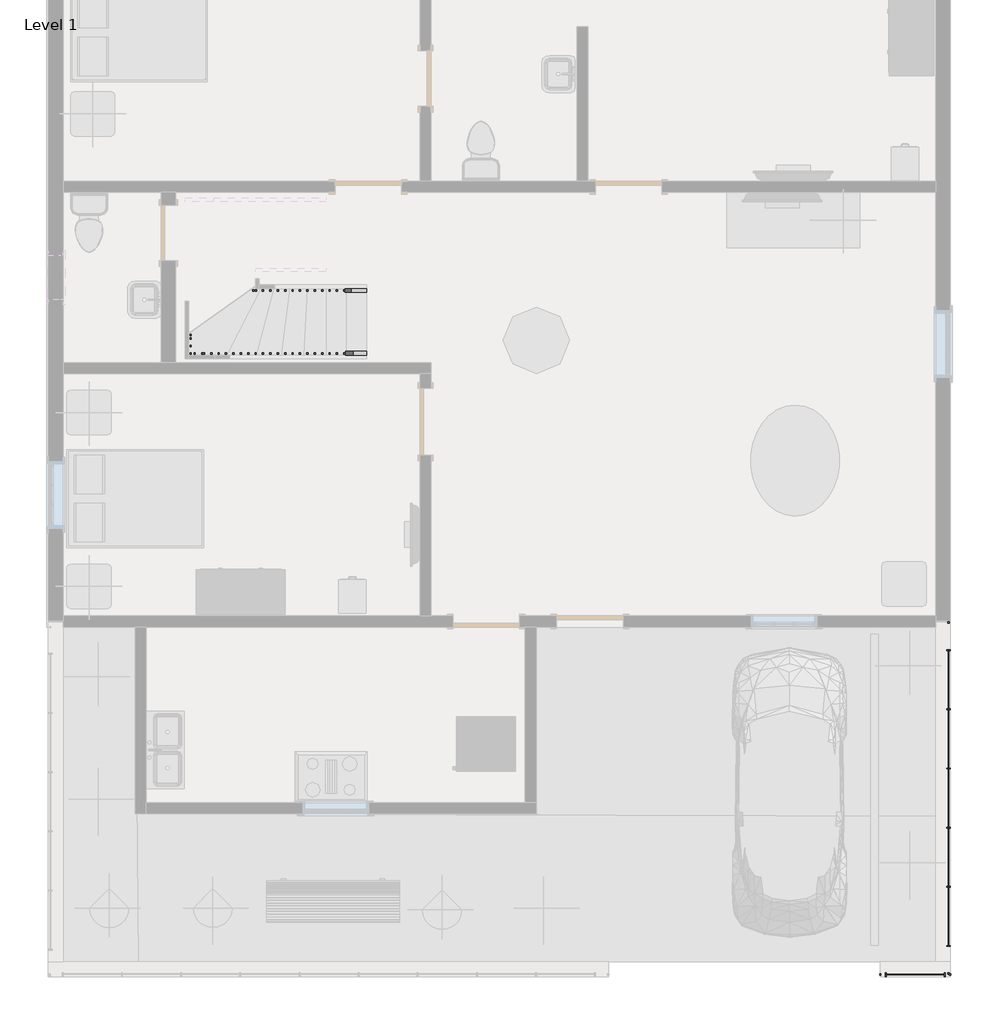
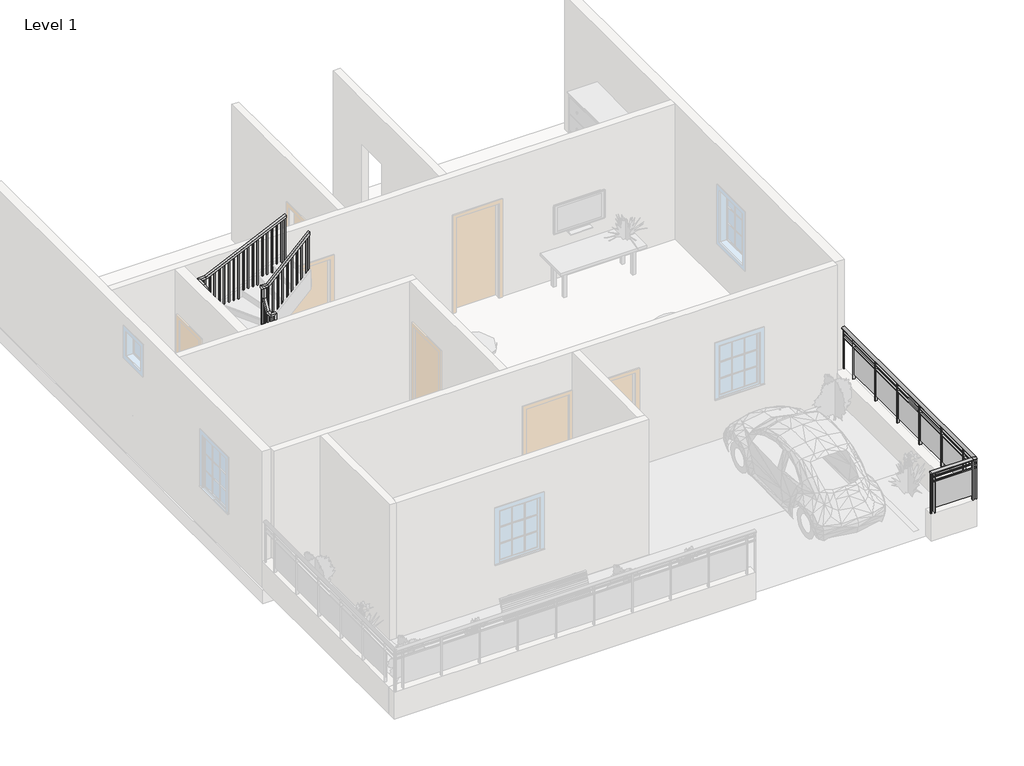
# One storey, part 2 of 3: 4 railings.
"""IFC4 building model written with IfcOpenShell, lengths in millimetres."""

from ifc_helpers import new_model, si_unit, point, frame, origin, place, context, project, spatial, polyline, ellipse_curve, trimmed, outline, extrude, faceted_brep, element, save
from ifc_brep_helpers import plane_surface, extruded_surface, advanced_brep

model = new_model("IFC4")

# Units and contexts
model_context = context("Model", 3, world=origin())
ifc_project = project(units=[si_unit("LENGTHUNIT", "METRE", prefix="MILLI")], contexts=[model_context])

# Site, building, storey
site = spatial("IfcSite", under=ifc_project)
building = spatial("IfcBuilding", under=site)
storey = spatial("IfcBuildingStorey", under=building, Name="Level 1", Elevation=0.0)

# Railings
placement = place(None, origin())
element("IfcRailing", 1, ObjectType="Glass Panel - Bottom Fill", at=placement, inside=storey, context=model_context, shape_type="SolidModel", body=[
    advanced_brep(
    [(-2180.6402453, -2817.8883114, 1524.0), (-2180.6402453, -2894.0883114, 1524.0), (-1215.4402453, -2817.8883114, 1524.0), (-1215.4402453, -2894.0883114, 1524.0)],
    [
        (0, 1, ellipse_curve(frame((-2180.6402453, -2855.9883114, 1524.0), z_axis=(-1.0, 0.0, 0.0), x_axis=(0.0, -1.0, 0.0)), 38.1, 28.575)),
        (1, 0, ellipse_curve(frame((-2180.6402453, -2855.9883114, 1524.0), z_axis=(-1.0, 0.0, 0.0), x_axis=(0.0, -1.0, 0.0)), 38.1, 28.575)),
        (2, 3, ellipse_curve(frame((-1215.4402453, -2855.9883114, 1524.0), z_axis=(1.0, 0.0, 0.0), x_axis=(0.0, -1.0, 0.0)), 38.1, 28.575)),
        (3, 2, ellipse_curve(frame((-1215.4402453, -2855.9883114, 1524.0), z_axis=(1.0, 0.0, 0.0), x_axis=(0.0, -1.0, 0.0)), 38.1, 28.575)),
        (0, 2),
        (3, 1),
    ],
    [
        plane_surface(frame((-2180.6402453, -2855.9883114, 1524.0), z_axis=(-1.0, 0.0, 0.0), x_axis=(0.0, 1.0, 0.0))),
        plane_surface(frame((-1215.4402453, -2855.9883114, 1524.0), z_axis=(1.0, 0.0, 0.0), x_axis=(0.0, 1.0, 0.0))),
        extruded_surface(trimmed(ellipse_curve(frame((-1215.4402453, -2855.9883114, 1524.0), z_axis=(-1.0, 0.0, 0.0), x_axis=(0.0, -1.0, 0.0)), 38.1, 28.575), [point((-1215.4402453, -2817.8883114, 1524.0))], [point((-1215.4402453, -2894.0883114, 1524.0))], True, "CARTESIAN"), (-965.2, 0.0, 0.0), 965.2),
        extruded_surface(trimmed(ellipse_curve(frame((-1215.4402453, -2855.9883114, 1524.0), z_axis=(-1.0, 0.0, 0.0), x_axis=(0.0, -1.0, 0.0)), 38.1, 28.575), [point((-1215.4402453, -2894.0883114, 1524.0))], [point((-1215.4402453, -2817.8883114, 1524.0))], True, "CARTESIAN"), (-965.2, 0.0, 0.0), 965.2),
    ],
    [
        (0, [[1, 2]]),
        (1, [[3, 4]]),
        (2, [[-1, 5, -4, 6]]),
        (3, [[-2, -6, -3, -5]]),
    ],
),
    extrude(outline(polyline([(-2180.6402453, -2868.6883114), (-2180.6402453, -2843.2883114), (-1215.4402453, -2843.2883114), (-1215.4402453, -2868.6883114), (-2180.6402453, -2868.6883114)])), frame((0.0, 0.0, 1409.7), z_axis=(0.0, 0.0, 1.0), x_axis=(1.0, 0.0, 0.0)), (0.0, 0.0, 1.0), 25.4),
    extrude(outline(polyline([(-2180.6402453, -2868.6883114), (-2180.6402453, -2843.2883114), (-1215.4402453, -2843.2883114), (-1215.4402453, -2868.6883114), (-2180.6402453, -2868.6883114)])), frame((0.0, 0.0, 1308.1), z_axis=(0.0, 0.0, 1.0), x_axis=(1.0, 0.0, 0.0)), (0.0, 0.0, 1.0), 25.4),
    extrude(outline(polyline([(-1297.9902453, -2881.3883114), (-1297.9902453, -2830.5883114), (-1285.2902453, -2830.5883114), (-1285.2902453, -2881.3883114), (-1297.9902453, -2881.3883114)])), frame((0.0, 0.0, 609.6), z_axis=(0.0, 0.0, 1.0), x_axis=(1.0, 0.0, 0.0)), (0.0, 0.0, 1.0), 885.6788223),
    extrude(outline(polyline([(-2104.4402453, -2849.4531544), (-1291.6402453, -2849.4531544), (-1291.6402453, -2855.8031544), (-2104.4402453, -2855.8031544), (-2104.4402453, -2849.4531544)])), frame((0.0, 0.0, 711.2), z_axis=(0.0, 0.0, 1.0), x_axis=(1.0, 0.0, 0.0)), (0.0, 0.0, 1.0), 596.9),
    extrude(outline(polyline([(-2110.7902453, -2881.3883114), (-2110.7902453, -2830.5883114), (-2098.0902453, -2830.5883114), (-2098.0902453, -2881.3883114), (-2110.7902453, -2881.3883114)])), frame((0.0, 0.0, 609.6), z_axis=(0.0, 0.0, 1.0), x_axis=(1.0, 0.0, 0.0)), (0.0, 0.0, 1.0), 885.6788223),
    extrude(outline(polyline([(-1228.1402453, -2865.5133114), (-1228.1402453, -2846.4633114), (-1209.0902453, -2846.4633114), (-1209.0902453, -2865.5133114), (-1228.1402453, -2865.5133114)])), frame((0.0, 0.0, 609.6), z_axis=(0.0, 0.0, 1.0), x_axis=(1.0, 0.0, 0.0)), (0.0, 0.0, 1.0), 885.6788223),
    extrude(outline(polyline([(-2186.9902453, -2865.5133114), (-2186.9902453, -2846.4633114), (-2167.9402453, -2846.4633114), (-2167.9402453, -2865.5133114), (-2186.9902453, -2865.5133114)])), frame((0.0, 0.0, 609.6), z_axis=(0.0, 0.0, 1.0), x_axis=(1.0, 0.0, 0.0)), (0.0, 0.0, 1.0), 885.6788223),
])
element("IfcRailing", 2, ObjectType="Glass Panel - Bottom Fill", at=placement, inside=storey, context=model_context, shape_type="SolidModel", body=[
    advanced_brep(
    [(-1202.7402453, 1982.7116886, 1524.0), (-1278.9402453, 1982.7116886, 1524.0), (-1202.7402453, -2843.2883114, 1524.0), (-1278.9402453, -2843.2883114, 1524.0)],
    [
        (0, 1, ellipse_curve(frame((-1240.8402453, 1982.7116886, 1524.0), z_axis=(0.0, 1.0, 0.0), x_axis=(-1.0, 0.0, 0.0)), 38.1, 28.575)),
        (1, 0, ellipse_curve(frame((-1240.8402453, 1982.7116886, 1524.0), z_axis=(0.0, 1.0, 0.0), x_axis=(-1.0, 0.0, 0.0)), 38.1, 28.575)),
        (2, 3, ellipse_curve(frame((-1240.8402453, -2843.2883114, 1524.0), z_axis=(0.0, -1.0, 0.0), x_axis=(-1.0, 0.0, 0.0)), 38.1, 28.575)),
        (3, 2, ellipse_curve(frame((-1240.8402453, -2843.2883114, 1524.0), z_axis=(0.0, -1.0, 0.0), x_axis=(-1.0, 0.0, 0.0)), 38.1, 28.575)),
        (0, 2),
        (3, 1),
    ],
    [
        plane_surface(frame((-1240.8402453, 1982.7116886, 1524.0), z_axis=(0.0, 1.0, 0.0), x_axis=(0.0, 0.0, -1.0))),
        plane_surface(frame((-1240.8402453, -2843.2883114, 1524.0), z_axis=(0.0, -1.0, 0.0), x_axis=(0.0, 0.0, -1.0))),
        extruded_surface(trimmed(ellipse_curve(frame((-1240.8402453, -2843.2883114, 1524.0), z_axis=(0.0, 1.0, 0.0), x_axis=(-1.0, 0.0, 0.0)), 38.1, 28.575), [point((-1202.7402453, -2843.2883114, 1524.0))], [point((-1278.9402453, -2843.2883114, 1524.0))], True, "CARTESIAN"), (0.0, 4826.0, 0.0), 4826.0),
        extruded_surface(trimmed(ellipse_curve(frame((-1240.8402453, -2843.2883114, 1524.0), z_axis=(0.0, 1.0, 0.0), x_axis=(-1.0, 0.0, 0.0)), 38.1, 28.575), [point((-1278.9402453, -2843.2883114, 1524.0))], [point((-1202.7402453, -2843.2883114, 1524.0))], True, "CARTESIAN"), (0.0, 4826.0, 0.0), 4826.0),
    ],
    [
        (0, [[1, 2]]),
        (1, [[3, 4]]),
        (2, [[-1, 5, -4, 6]]),
        (3, [[-2, -6, -3, -5]]),
    ],
),
    extrude(outline(polyline([(-1253.5402453, 1982.7116886), (-1228.1402453, 1982.7116886), (-1228.1402453, -2843.2883114), (-1253.5402453, -2843.2883114), (-1253.5402453, 1982.7116886)])), frame((0.0, 0.0, 1409.7), z_axis=(0.0, 0.0, 1.0), x_axis=(1.0, 0.0, 0.0)), (0.0, 0.0, 1.0), 25.4),
    extrude(outline(polyline([(-1253.5402453, 1982.7116886), (-1228.1402453, 1982.7116886), (-1228.1402453, -2843.2883114), (-1253.5402453, -2843.2883114), (-1253.5402453, 1982.7116886)])), frame((0.0, 0.0, 1308.1), z_axis=(0.0, 0.0, 1.0), x_axis=(1.0, 0.0, 0.0)), (0.0, 0.0, 1.0), 25.4),
    extrude(outline(polyline([(-1266.2402453, -2455.9383114), (-1215.4402453, -2455.9383114), (-1215.4402453, -2468.6383114), (-1266.2402453, -2468.6383114), (-1266.2402453, -2455.9383114)])), frame((0.0, 0.0, 609.6), z_axis=(0.0, 0.0, 1.0), x_axis=(1.0, 0.0, 0.0)), (0.0, 0.0, 1.0), 885.6788223),
    extrude(outline(polyline([(-1234.3050883, -1649.4883114), (-1234.3050883, -2462.2883114), (-1240.6550883, -2462.2883114), (-1240.6550883, -1649.4883114), (-1234.3050883, -1649.4883114)])), frame((0.0, 0.0, 711.2), z_axis=(0.0, 0.0, 1.0), x_axis=(1.0, 0.0, 0.0)), (0.0, 0.0, 1.0), 596.9),
    extrude(outline(polyline([(-1266.2402453, -1643.1383114), (-1215.4402453, -1643.1383114), (-1215.4402453, -1655.8383114), (-1266.2402453, -1655.8383114), (-1266.2402453, -1643.1383114)])), frame((0.0, 0.0, 609.6), z_axis=(0.0, 0.0, 1.0), x_axis=(1.0, 0.0, 0.0)), (0.0, 0.0, 1.0), 885.6788223),
    extrude(outline(polyline([(-1234.3050883, -836.6883114), (-1234.3050883, -1649.4883114), (-1240.6550883, -1649.4883114), (-1240.6550883, -836.6883114), (-1234.3050883, -836.6883114)])), frame((0.0, 0.0, 711.2), z_axis=(0.0, 0.0, 1.0), x_axis=(1.0, 0.0, 0.0)), (0.0, 0.0, 1.0), 596.9),
    extrude(outline(polyline([(-1266.2402453, -830.3383114), (-1215.4402453, -830.3383114), (-1215.4402453, -843.0383114), (-1266.2402453, -843.0383114), (-1266.2402453, -830.3383114)])), frame((0.0, 0.0, 609.6), z_axis=(0.0, 0.0, 1.0), x_axis=(1.0, 0.0, 0.0)), (0.0, 0.0, 1.0), 885.6788223),
    extrude(outline(polyline([(-1234.3050883, -23.8883114), (-1234.3050883, -836.6883114), (-1240.6550883, -836.6883114), (-1240.6550883, -23.8883114), (-1234.3050883, -23.8883114)])), frame((0.0, 0.0, 711.2), z_axis=(0.0, 0.0, 1.0), x_axis=(1.0, 0.0, 0.0)), (0.0, 0.0, 1.0), 596.9),
    extrude(outline(polyline([(-1266.2402453, -17.5383114), (-1215.4402453, -17.5383114), (-1215.4402453, -30.2383114), (-1266.2402453, -30.2383114), (-1266.2402453, -17.5383114)])), frame((0.0, 0.0, 609.6), z_axis=(0.0, 0.0, 1.0), x_axis=(1.0, 0.0, 0.0)), (0.0, 0.0, 1.0), 885.6788223),
    extrude(outline(polyline([(-1234.3050883, 788.9116886), (-1234.3050883, -23.8883114), (-1240.6550883, -23.8883114), (-1240.6550883, 788.9116886), (-1234.3050883, 788.9116886)])), frame((0.0, 0.0, 711.2), z_axis=(0.0, 0.0, 1.0), x_axis=(1.0, 0.0, 0.0)), (0.0, 0.0, 1.0), 596.9),
    extrude(outline(polyline([(-1266.2402453, 795.2616886), (-1215.4402453, 795.2616886), (-1215.4402453, 782.5616886), (-1266.2402453, 782.5616886), (-1266.2402453, 795.2616886)])), frame((0.0, 0.0, 609.6), z_axis=(0.0, 0.0, 1.0), x_axis=(1.0, 0.0, 0.0)), (0.0, 0.0, 1.0), 885.6788223),
    extrude(outline(polyline([(-1234.3050883, 1601.7116886), (-1234.3050883, 788.9116886), (-1240.6550883, 788.9116886), (-1240.6550883, 1601.7116886), (-1234.3050883, 1601.7116886)])), frame((0.0, 0.0, 711.2), z_axis=(0.0, 0.0, 1.0), x_axis=(1.0, 0.0, 0.0)), (0.0, 0.0, 1.0), 596.9),
    extrude(outline(polyline([(-1266.2402453, 1608.0616886), (-1215.4402453, 1608.0616886), (-1215.4402453, 1595.3616886), (-1266.2402453, 1595.3616886), (-1266.2402453, 1608.0616886)])), frame((0.0, 0.0, 609.6), z_axis=(0.0, 0.0, 1.0), x_axis=(1.0, 0.0, 0.0)), (0.0, 0.0, 1.0), 885.6788223),
    extrude(outline(polyline([(-1250.3652453, -2830.5883114), (-1231.3152453, -2830.5883114), (-1231.3152453, -2849.6383114), (-1250.3652453, -2849.6383114), (-1250.3652453, -2830.5883114)])), frame((0.0, 0.0, 609.6), z_axis=(0.0, 0.0, 1.0), x_axis=(1.0, 0.0, 0.0)), (0.0, 0.0, 1.0), 885.6788223),
    extrude(outline(polyline([(-1250.3652453, 1989.0616886), (-1231.3152453, 1989.0616886), (-1231.3152453, 1970.0116886), (-1250.3652453, 1970.0116886), (-1250.3652453, 1989.0616886)])), frame((0.0, 0.0, 609.6), z_axis=(0.0, 0.0, 1.0), x_axis=(1.0, 0.0, 0.0)), (0.0, 0.0, 1.0), 885.6788223),
])
element("IfcRailing", 3, ObjectType="Handrail - Rectangular", at=placement, inside=storey, context=model_context, shape_type="SolidModel", body=[
    faceted_brep([(-9238.1085535, 6516.6116886, 1025.2529681), (-9238.1085535, 6516.6116886, 959.7067088), (-9238.1085535, 6567.4116886, 959.7067088), (-9238.1085535, 6567.4116886, 1025.2529681), (-10689.6402453, 6516.6116886, 2208.7848338), (-10740.4402453, 6516.6116886, 2184.659247), (-10740.4402453, 6567.4116886, 2184.659247), (-10689.6402453, 6567.4116886, 2208.7848338), (-10689.6402453, 6516.6116886, 2414.6281882), (-10740.4402453, 6516.6116886, 2363.8281882), (-10740.4402453, 6567.4116886, 2363.8281882), (-10689.6402453, 6567.4116886, 2414.6281882), (-10816.6402453, 6516.6116886, 2414.6281882), (-10816.6402453, 6516.6116886, 2363.8281882), (-10765.8402453, 6567.4116886, 2363.8281882), (-10765.8402453, 6567.4116886, 2414.6281882), (-10816.6402453, 6643.6116886, 2414.6281882), (-10816.6402453, 6672.7330225, 2363.8281882), (-10765.8402453, 6672.7330225, 2363.8281882), (-10765.8402453, 6643.6116886, 2414.6281882), (-10816.6402453, 6770.6116886, 2631.5051451), (-10816.6402453, 6821.4116886, 2617.7256424), (-10765.8402453, 6821.4116886, 2617.7256424), (-10765.8402453, 6770.6116886, 2631.5051451), (-10816.6402453, 6770.6116886, 2849.930498), (-10816.6402453, 6821.4116886, 2799.130498), (-10765.8402453, 6821.4116886, 2799.130498), (-10765.8402453, 6770.6116886, 2849.930498), (-10816.6402453, 6897.6116886, 2849.930498), (-10816.6402453, 6897.6116886, 2799.130498), (-10765.8402453, 6846.8116886, 2799.130498), (-10765.8402453, 6846.8116886, 2849.930498), (-10689.6402453, 6897.6116886, 2849.930498), (-10668.8144223, 6897.6116886, 2799.130498), (-10668.8144223, 6846.8116886, 2799.130498), (-10689.6402453, 6846.8116886, 2849.930498), (-9796.9085535, 6897.6116886, 3729.7628764), (-9796.9085535, 6846.8116886, 3729.7628764), (-9796.9085535, 6846.8116886, 3658.4379712), (-9796.9085535, 6897.6116886, 3658.4379712)], [[[0, 1, 2, 3]], [[1, 0, 4, 5]], [[2, 1, 5, 6]], [[3, 2, 6, 7]], [[0, 3, 7, 4]], [[5, 4, 8, 9]], [[6, 5, 9, 10]], [[7, 6, 10, 11]], [[4, 7, 11, 8]], [[9, 8, 12, 13]], [[10, 9, 13, 14]], [[11, 10, 14, 15]], [[8, 11, 15, 12]], [[13, 12, 16, 17]], [[14, 13, 17, 18]], [[15, 14, 18, 19]], [[12, 15, 19, 16]], [[17, 16, 20, 21]], [[18, 17, 21, 22]], [[19, 18, 22, 23]], [[16, 19, 23, 20]], [[21, 20, 24, 25]], [[22, 21, 25, 26]], [[23, 22, 26, 27]], [[20, 23, 27, 24]], [[25, 24, 28, 29]], [[26, 25, 29, 30]], [[27, 26, 30, 31]], [[24, 27, 31, 28]], [[29, 28, 32, 33]], [[30, 29, 33, 34]], [[31, 30, 34, 35]], [[28, 31, 35, 32]], [[36, 37, 38, 39]], [[33, 32, 36, 39]], [[34, 33, 39, 38]], [[35, 34, 38, 37]], [[32, 35, 37, 36]]]),
    extrude(outline(polyline([(3616.6526879, -9839.3064551), (3597.8779463, -9858.3564551), (2540.0, -9858.3564551), (2540.0, -9839.3064551), (3616.6526879, -9839.3064551)])), frame((0.0, 6862.6866886, 0.0), z_axis=(0.0, 1.0, 0.0), x_axis=(0.0, 0.0, 1.0)), (0.0, 0.0, 1.0), 19.05),
    extrude(outline(polyline([(3516.5207329, -9940.9064551), (3497.7459913, -9959.9564551), (2540.0, -9959.9564551), (2540.0, -9940.9064551), (3516.5207329, -9940.9064551)])), frame((0.0, 6862.6866886, 0.0), z_axis=(0.0, 1.0, 0.0), x_axis=(0.0, 0.0, 1.0)), (0.0, 0.0, 1.0), 19.05),
    extrude(outline(polyline([(3416.3887778, -10042.5064551), (3397.6140362, -10061.5564551), (2540.0, -10061.5564551), (2540.0, -10042.5064551), (3416.3887778, -10042.5064551)])), frame((0.0, 6862.6866886, 0.0), z_axis=(0.0, 1.0, 0.0), x_axis=(0.0, 0.0, 1.0)), (0.0, 0.0, 1.0), 19.05),
    extrude(outline(polyline([(3316.2568227, -10144.1064551), (3297.4820812, -10163.1564551), (2370.6666667, -10163.1564551), (2370.6666667, -10144.1064551), (3316.2568227, -10144.1064551)])), frame((0.0, 6862.6866886, 0.0), z_axis=(0.0, 1.0, 0.0), x_axis=(0.0, 0.0, 1.0)), (0.0, 0.0, 1.0), 19.05),
    extrude(outline(polyline([(3216.1248677, -10245.7064551), (3197.3501261, -10264.7564551), (2370.6666667, -10264.7564551), (2370.6666667, -10245.7064551), (3216.1248677, -10245.7064551)])), frame((0.0, 6862.6866886, 0.0), z_axis=(0.0, 1.0, 0.0), x_axis=(0.0, 0.0, 1.0)), (0.0, 0.0, 1.0), 19.05),
    extrude(outline(polyline([(3115.9929126, -10347.3064551), (3097.218171, -10366.3564551), (2201.3333333, -10366.3564551), (2201.3333333, -10347.3064551), (3115.9929126, -10347.3064551)])), frame((0.0, 6862.6866886, 0.0), z_axis=(0.0, 1.0, 0.0), x_axis=(0.0, 0.0, 1.0)), (0.0, 0.0, 1.0), 19.05),
    extrude(outline(polyline([(3015.8609575, -10448.9064551), (2997.086216, -10467.9564551), (2201.3333333, -10467.9564551), (2201.3333333, -10448.9064551), (3015.8609575, -10448.9064551)])), frame((0.0, 6862.6866886, 0.0), z_axis=(0.0, 1.0, 0.0), x_axis=(0.0, 0.0, 1.0)), (0.0, 0.0, 1.0), 19.05),
    extrude(outline(polyline([(2915.7290025, -10550.5064551), (2896.9542609, -10569.5564551), (2032.0, -10569.5564551), (2032.0, -10550.5064551), (2915.7290025, -10550.5064551)])), frame((0.0, 6862.6866886, 0.0), z_axis=(0.0, 1.0, 0.0), x_axis=(0.0, 0.0, 1.0)), (0.0, 0.0, 1.0), 19.05),
    extrude(outline(polyline([(2815.5970474, -10652.1064551), (2796.8223058, -10671.1564551), (2032.0, -10671.1564551), (2032.0, -10652.1064551), (2815.5970474, -10652.1064551)])), frame((0.0, 6862.6866886, 0.0), z_axis=(0.0, 1.0, 0.0), x_axis=(0.0, 0.0, 1.0)), (0.0, 0.0, 1.0), 19.05),
    extrude(outline(polyline([(6750.4725924, 2496.5834745), (6769.5225924, 2529.115018), (6769.5225924, 1524.0), (6750.4725924, 1524.0), (6750.4725924, 2496.5834745)])), frame((-10800.7652453, 0.0, 0.0), z_axis=(1.0, 0.0, 0.0), x_axis=(0.0, 1.0, 0.0)), (0.0, 0.0, 1.0), 19.05),
    extrude(outline(polyline([(6648.8725924, 2323.0819089), (6667.9225924, 2355.6134525), (6667.9225924, 1524.0), (6648.8725924, 1524.0), (6648.8725924, 2323.0819089)])), frame((-10800.7652453, 0.0, 0.0), z_axis=(1.0, 0.0, 0.0), x_axis=(0.0, 1.0, 0.0)), (0.0, 0.0, 1.0), 19.05),
    extrude(outline(polyline([(2111.7191617, -10650.9835535), (2127.2519138, -10670.0335535), (1016.0, -10670.0335535), (1016.0, -10650.9835535), (2111.7191617, -10650.9835535)])), frame((0.0, 6532.4866886, 0.0), z_axis=(0.0, 1.0, 0.0), x_axis=(0.0, 0.0, 1.0)), (0.0, 0.0, 1.0), 19.05),
    extrude(outline(polyline([(2028.8778167, -10549.3835535), (2044.4105689, -10568.4335535), (1016.0, -10568.4335535), (1016.0, -10549.3835535), (2028.8778167, -10549.3835535)])), frame((0.0, 6532.4866886, 0.0), z_axis=(0.0, 1.0, 0.0), x_axis=(0.0, 0.0, 1.0)), (0.0, 0.0, 1.0), 19.05),
    extrude(outline(polyline([(1946.0364718, -10447.7835535), (1961.569224, -10466.8335535), (846.6666667, -10466.8335535), (846.6666667, -10447.7835535), (1946.0364718, -10447.7835535)])), frame((0.0, 6532.4866886, 0.0), z_axis=(0.0, 1.0, 0.0), x_axis=(0.0, 0.0, 1.0)), (0.0, 0.0, 1.0), 19.05),
    extrude(outline(polyline([(1863.1951269, -10346.1835535), (1878.7278791, -10365.2335535), (846.6666667, -10365.2335535), (846.6666667, -10346.1835535), (1863.1951269, -10346.1835535)])), frame((0.0, 6532.4866886, 0.0), z_axis=(0.0, 1.0, 0.0), x_axis=(0.0, 0.0, 1.0)), (0.0, 0.0, 1.0), 19.05),
    extrude(outline(polyline([(1780.353782, -10244.5835535), (1795.8865341, -10263.6335535), (677.3333333, -10263.6335535), (677.3333333, -10244.5835535), (1780.353782, -10244.5835535)])), frame((0.0, 6532.4866886, 0.0), z_axis=(0.0, 1.0, 0.0), x_axis=(0.0, 0.0, 1.0)), (0.0, 0.0, 1.0), 19.05),
    extrude(outline(polyline([(1697.5124371, -10142.9835535), (1713.0451892, -10162.0335535), (677.3333333, -10162.0335535), (677.3333333, -10142.9835535), (1697.5124371, -10142.9835535)])), frame((0.0, 6532.4866886, 0.0), z_axis=(0.0, 1.0, 0.0), x_axis=(0.0, 0.0, 1.0)), (0.0, 0.0, 1.0), 19.05),
    extrude(outline(polyline([(1614.6710921, -10041.3835535), (1630.2038443, -10060.4335535), (508.0, -10060.4335535), (508.0, -10041.3835535), (1614.6710921, -10041.3835535)])), frame((0.0, 6532.4866886, 0.0), z_axis=(0.0, 1.0, 0.0), x_axis=(0.0, 0.0, 1.0)), (0.0, 0.0, 1.0), 19.05),
    extrude(outline(polyline([(1531.8297472, -9939.7835535), (1547.3624994, -9958.8335535), (508.0, -9958.8335535), (508.0, -9939.7835535), (1531.8297472, -9939.7835535)])), frame((0.0, 6532.4866886, 0.0), z_axis=(0.0, 1.0, 0.0), x_axis=(0.0, 0.0, 1.0)), (0.0, 0.0, 1.0), 19.05),
    extrude(outline(polyline([(1448.9884023, -9838.1835535), (1464.5211545, -9857.2335535), (508.0, -9857.2335535), (508.0, -9838.1835535), (1448.9884023, -9838.1835535)])), frame((0.0, 6532.4866886, 0.0), z_axis=(0.0, 1.0, 0.0), x_axis=(0.0, 0.0, 1.0)), (0.0, 0.0, 1.0), 19.05),
    extrude(outline(polyline([(1366.1470574, -9736.5835535), (1381.6798095, -9755.6335535), (338.6666667, -9755.6335535), (338.6666667, -9736.5835535), (1366.1470574, -9736.5835535)])), frame((0.0, 6532.4866886, 0.0), z_axis=(0.0, 1.0, 0.0), x_axis=(0.0, 0.0, 1.0)), (0.0, 0.0, 1.0), 19.05),
    extrude(outline(polyline([(1283.3057124, -9634.9835535), (1298.8384646, -9654.0335535), (338.6666667, -9654.0335535), (338.6666667, -9634.9835535), (1283.3057124, -9634.9835535)])), frame((0.0, 6532.4866886, 0.0), z_axis=(0.0, 1.0, 0.0), x_axis=(0.0, 0.0, 1.0)), (0.0, 0.0, 1.0), 19.05),
    extrude(outline(polyline([(1200.4643675, -9533.3835535), (1215.9971197, -9552.4335535), (338.6666667, -9552.4335535), (338.6666667, -9533.3835535), (1200.4643675, -9533.3835535)])), frame((0.0, 6532.4866886, 0.0), z_axis=(0.0, 1.0, 0.0), x_axis=(0.0, 0.0, 1.0)), (0.0, 0.0, 1.0), 19.05),
    extrude(outline(polyline([(1117.6230226, -9431.7835535), (1133.1557748, -9450.8335535), (169.3333333, -9450.8335535), (169.3333333, -9431.7835535), (1117.6230226, -9431.7835535)])), frame((0.0, 6532.4866886, 0.0), z_axis=(0.0, 1.0, 0.0), x_axis=(0.0, 0.0, 1.0)), (0.0, 0.0, 1.0), 19.05),
    extrude(outline(polyline([(1034.7816777, -9330.1835535), (1050.3144298, -9349.2335535), (169.3333333, -9349.2335535), (169.3333333, -9330.1835535), (1034.7816777, -9330.1835535)])), frame((0.0, 6532.4866886, 0.0), z_axis=(0.0, 1.0, 0.0), x_axis=(0.0, 0.0, 1.0)), (0.0, 0.0, 1.0), 19.05),
    extrude(outline(polyline([(-10772.7564551, 6862.6866886), (-10772.7564551, 6881.7366886), (-10753.7064551, 6881.7366886), (-10753.7064551, 6862.6866886), (-10772.7564551, 6862.6866886)])), frame((0.0, 0.0, 1862.6666667), z_axis=(0.0, 0.0, 1.0), x_axis=(1.0, 0.0, 0.0)), (0.0, 0.0, 1.0), 936.4638313),
    extrude(outline(polyline([(-10781.7152453, 6862.6866886), (-10800.7652453, 6862.6866886), (-10800.7652453, 6881.7366886), (-10781.7152453, 6881.7366886), (-10781.7152453, 6862.6866886)])), frame((0.0, 0.0, 1862.6666667), z_axis=(0.0, 0.0, 1.0), x_axis=(1.0, 0.0, 0.0)), (0.0, 0.0, 1.0), 936.4638313),
    extrude(outline(polyline([(-10781.7152453, 6846.5221375), (-10800.7652453, 6846.5221375), (-10800.7652453, 6865.5721375), (-10781.7152453, 6865.5721375), (-10781.7152453, 6846.5221375)])), frame((0.0, 0.0, 1693.3333333), z_axis=(0.0, 0.0, 1.0), x_axis=(1.0, 0.0, 0.0)), (0.0, 0.0, 1.0), 1105.7971646),
    extrude(outline(polyline([(-10781.7152453, 6547.2725924), (-10800.7652453, 6547.2725924), (-10800.7652453, 6566.3225924), (-10781.7152453, 6566.3225924), (-10781.7152453, 6547.2725924)])), frame((0.0, 0.0, 1354.6666667), z_axis=(0.0, 0.0, 1.0), x_axis=(1.0, 0.0, 0.0)), (0.0, 0.0, 1.0), 1009.1615215),
    extrude(outline(polyline([(-10781.7152453, 6551.5366886), (-10781.7152453, 6532.4866886), (-10800.7652453, 6532.4866886), (-10800.7652453, 6551.5366886), (-10781.7152453, 6551.5366886)])), frame((0.0, 0.0, 1185.3333333), z_axis=(0.0, 0.0, 1.0), x_axis=(1.0, 0.0, 0.0)), (0.0, 0.0, 1.0), 1178.4948549),
    extrude(outline(polyline([(-10750.747889, 6551.5366886), (-10750.747889, 6532.4866886), (-10769.797889, 6532.4866886), (-10769.797889, 6551.5366886), (-10750.747889, 6551.5366886)])), frame((0.0, 0.0, 1185.3333333), z_axis=(0.0, 0.0, 1.0), x_axis=(1.0, 0.0, 0.0)), (0.0, 0.0, 1.0), 1178.4948549),
    extrude(outline(polyline([(3658.4379712, -9796.9085535), (3639.6632296, -9815.9585535), (2540.0, -9815.9585535), (2540.0, -9796.9085535), (3658.4379712, -9796.9085535)])), frame((0.0, 6862.6866886, 0.0), z_axis=(0.0, 1.0, 0.0), x_axis=(0.0, 0.0, 1.0)), (0.0, 0.0, 1.0), 19.05),
    extrude(outline(polyline([(959.7067088, -9238.1085535), (975.239461, -9257.1585535), (169.3333333, -9257.1585535), (169.3333333, -9238.1085535), (959.7067088, -9238.1085535)])), frame((0.0, 6532.4866886, 0.0), z_axis=(0.0, 1.0, 0.0), x_axis=(0.0, 0.0, 1.0)), (0.0, 0.0, 1.0), 19.05),
])
element("IfcRailing", 4, ObjectType="Handrail - Rectangular", at=placement, inside=storey, context=model_context, shape_type="SolidModel", body=[
    faceted_brep([(-9238.1085535, 5653.0116886, 1109.0771751), (-9238.1085535, 5653.0116886, 1051.9280057), (-9238.1085535, 5703.8116886, 1051.9280057), (-9238.1085535, 5703.8116886, 1109.0771751), (-11498.0904099, 5653.0116886, 2273.7644996), (-11510.4104612, 5653.0116886, 2222.9644996), (-11510.4104612, 5703.8116886, 2222.9644996), (-11498.0904099, 5703.8116886, 2273.7644996), (-11680.2402453, 5653.0116886, 2273.7644996), (-11680.2402453, 5653.0116886, 2222.9644996), (-11629.4402453, 5703.8116886, 2222.9644996), (-11629.4402453, 5703.8116886, 2273.7644996), (-11680.2402453, 5930.1656412, 2273.7644996), (-11680.2402453, 5938.1162174, 2222.9644996), (-11629.4402453, 5938.1162174, 2222.9644996), (-11629.4402453, 5930.1656412, 2273.7644996), (-11680.2402453, 7520.0814957, 2783.9279392), (-11680.2402453, 7528.0320718, 2733.1279392), (-11629.4402453, 7528.0320718, 2733.1279392), (-11629.4402453, 7520.0814957, 2783.9279392), (-11680.2402453, 7761.2116886, 2783.9279392), (-11680.2402453, 7761.2116886, 2733.1279392), (-11629.4402453, 7710.4116886, 2733.1279392), (-11629.4402453, 7710.4116886, 2783.9279392), (-11507.1175877, 7761.2116886, 2783.9279392), (-11495.805433, 7761.2116886, 2733.1279392), (-11495.805433, 7710.4116886, 2733.1279392), (-11507.1175877, 7710.4116886, 2783.9279392), (-9796.9085535, 7761.2116886, 3585.3258533), (-9796.9085535, 7710.4116886, 3585.3258533), (-9796.9085535, 7710.4116886, 3529.2250176), (-9796.9085535, 7761.2116886, 3529.2250176)], [[[0, 1, 2, 3]], [[1, 0, 4, 5]], [[2, 1, 5, 6]], [[3, 2, 6, 7]], [[0, 3, 7, 4]], [[5, 4, 8, 9]], [[6, 5, 9, 10]], [[7, 6, 10, 11]], [[4, 7, 11, 8]], [[9, 8, 12, 13]], [[10, 9, 13, 14]], [[11, 10, 14, 15]], [[8, 11, 15, 12]], [[13, 12, 16, 17]], [[14, 13, 17, 18]], [[15, 14, 18, 19]], [[12, 15, 19, 16]], [[17, 16, 20, 21]], [[18, 17, 21, 22]], [[19, 18, 22, 23]], [[16, 19, 23, 20]], [[21, 20, 24, 25]], [[22, 21, 25, 26]], [[23, 22, 26, 27]], [[20, 23, 27, 24]], [[28, 29, 30, 31]], [[25, 24, 28, 31]], [[26, 25, 31, 30]], [[27, 26, 30, 29]], [[24, 27, 29, 28]]]),
    extrude(outline(polyline([(3485.1141416, -9891.0425877), (2540.0, -9891.0425877), (2540.0, -9871.9925877), (3494.0409043, -9871.9925877), (3485.1141416, -9891.0425877)])), frame((0.0, 7726.2866886, 0.0), z_axis=(0.0, 1.0, 0.0), x_axis=(0.0, 0.0, 1.0)), (0.0, 0.0, 1.0), 19.05),
    extrude(outline(polyline([(3437.5047404, -9992.6425877), (2540.0, -9992.6425877), (2540.0, -9973.5925877), (3446.4315031, -9973.5925877), (3437.5047404, -9992.6425877)])), frame((0.0, 7726.2866886, 0.0), z_axis=(0.0, 1.0, 0.0), x_axis=(0.0, 0.0, 1.0)), (0.0, 0.0, 1.0), 19.05),
    extrude(outline(polyline([(3389.8953392, -10094.2425877), (2370.6666667, -10094.2425877), (2370.6666667, -10075.1925877), (3398.8221019, -10075.1925877), (3389.8953392, -10094.2425877)])), frame((0.0, 7726.2866886, 0.0), z_axis=(0.0, 1.0, 0.0), x_axis=(0.0, 0.0, 1.0)), (0.0, 0.0, 1.0), 19.05),
    extrude(outline(polyline([(3342.2859379, -10195.8425877), (2370.6666667, -10195.8425877), (2370.6666667, -10176.7925877), (3351.2127007, -10176.7925877), (3342.2859379, -10195.8425877)])), frame((0.0, 7726.2866886, 0.0), z_axis=(0.0, 1.0, 0.0), x_axis=(0.0, 0.0, 1.0)), (0.0, 0.0, 1.0), 19.05),
    extrude(outline(polyline([(3294.6765367, -10297.4425877), (2370.6666667, -10297.4425877), (2370.6666667, -10278.3925877), (3303.6032995, -10278.3925877), (3294.6765367, -10297.4425877)])), frame((0.0, 7726.2866886, 0.0), z_axis=(0.0, 1.0, 0.0), x_axis=(0.0, 0.0, 1.0)), (0.0, 0.0, 1.0), 19.05),
    extrude(outline(polyline([(3247.0671355, -10399.0425877), (2201.3333333, -10399.0425877), (2201.3333333, -10379.9925877), (3255.9938982, -10379.9925877), (3247.0671355, -10399.0425877)])), frame((0.0, 7726.2866886, 0.0), z_axis=(0.0, 1.0, 0.0), x_axis=(0.0, 0.0, 1.0)), (0.0, 0.0, 1.0), 19.05),
    extrude(outline(polyline([(3199.4577343, -10500.6425877), (2201.3333333, -10500.6425877), (2201.3333333, -10481.5925877), (3208.384497, -10481.5925877), (3199.4577343, -10500.6425877)])), frame((0.0, 7726.2866886, 0.0), z_axis=(0.0, 1.0, 0.0), x_axis=(0.0, 0.0, 1.0)), (0.0, 0.0, 1.0), 19.05),
    extrude(outline(polyline([(3151.8483331, -10602.2425877), (2201.3333333, -10602.2425877), (2201.3333333, -10583.1925877), (3160.7750958, -10583.1925877), (3151.8483331, -10602.2425877)])), frame((0.0, 7726.2866886, 0.0), z_axis=(0.0, 1.0, 0.0), x_axis=(0.0, 0.0, 1.0)), (0.0, 0.0, 1.0), 19.05),
    extrude(outline(polyline([(3104.2389319, -10703.8425877), (2201.3333333, -10703.8425877), (2201.3333333, -10684.7925877), (3113.1656946, -10684.7925877), (3104.2389319, -10703.8425877)])), frame((0.0, 7726.2866886, 0.0), z_axis=(0.0, 1.0, 0.0), x_axis=(0.0, 0.0, 1.0)), (0.0, 0.0, 1.0), 19.05),
    extrude(outline(polyline([(3056.6295307, -10805.4425877), (2032.0, -10805.4425877), (2032.0, -10786.3925877), (3065.5562934, -10786.3925877), (3056.6295307, -10805.4425877)])), frame((0.0, 7726.2866886, 0.0), z_axis=(0.0, 1.0, 0.0), x_axis=(0.0, 0.0, 1.0)), (0.0, 0.0, 1.0), 19.05),
    extrude(outline(polyline([(3009.0201294, -10907.0425877), (2032.0, -10907.0425877), (2032.0, -10887.9925877), (3017.9468922, -10887.9925877), (3009.0201294, -10907.0425877)])), frame((0.0, 7726.2866886, 0.0), z_axis=(0.0, 1.0, 0.0), x_axis=(0.0, 0.0, 1.0)), (0.0, 0.0, 1.0), 19.05),
    extrude(outline(polyline([(2961.4107282, -11008.6425877), (2032.0, -11008.6425877), (2032.0, -10989.5925877), (2970.3374909, -10989.5925877), (2961.4107282, -11008.6425877)])), frame((0.0, 7726.2866886, 0.0), z_axis=(0.0, 1.0, 0.0), x_axis=(0.0, 0.0, 1.0)), (0.0, 0.0, 1.0), 19.05),
    extrude(outline(polyline([(2913.801327, -11110.2425877), (2032.0, -11110.2425877), (2032.0, -11091.1925877), (2922.7280897, -11091.1925877), (2913.801327, -11110.2425877)])), frame((0.0, 7726.2866886, 0.0), z_axis=(0.0, 1.0, 0.0), x_axis=(0.0, 0.0, 1.0)), (0.0, 0.0, 1.0), 19.05),
    extrude(outline(polyline([(2866.1919258, -11211.8425877), (1862.6666667, -11211.8425877), (1862.6666667, -11192.7925877), (2875.1186885, -11192.7925877), (2866.1919258, -11211.8425877)])), frame((0.0, 7726.2866886, 0.0), z_axis=(0.0, 1.0, 0.0), x_axis=(0.0, 0.0, 1.0)), (0.0, 0.0, 1.0), 19.05),
    extrude(outline(polyline([(2818.5825246, -11313.4425877), (1862.6666667, -11313.4425877), (1862.6666667, -11294.3925877), (2827.5092873, -11294.3925877), (2818.5825246, -11313.4425877)])), frame((0.0, 7726.2866886, 0.0), z_axis=(0.0, 1.0, 0.0), x_axis=(0.0, 0.0, 1.0)), (0.0, 0.0, 1.0), 19.05),
    extrude(outline(polyline([(2770.9731234, -11415.0425877), (1862.6666667, -11415.0425877), (1862.6666667, -11395.9925877), (2779.8998861, -11395.9925877), (2770.9731234, -11415.0425877)])), frame((0.0, 7726.2866886, 0.0), z_axis=(0.0, 1.0, 0.0), x_axis=(0.0, 0.0, 1.0)), (0.0, 0.0, 1.0), 19.05),
    extrude(outline(polyline([(-11562.7652453, 7745.3366886), (-11543.7152453, 7745.3366886), (-11543.7152453, 7726.2866886), (-11562.7652453, 7726.2866886), (-11562.7652453, 7745.3366886)])), frame((0.0, 0.0, 1862.6666667), z_axis=(0.0, 0.0, 1.0), x_axis=(1.0, 0.0, 0.0)), (0.0, 0.0, 1.0), 870.4612726),
    extrude(outline(polyline([(-11664.3652453, 7713.7564957), (-11664.3652453, 7732.8064957), (-11645.3152453, 7732.8064957), (-11645.3152453, 7713.7564957), (-11664.3652453, 7713.7564957)])), frame((0.0, 0.0, 1862.6666667), z_axis=(0.0, 0.0, 1.0), x_axis=(1.0, 0.0, 0.0)), (0.0, 0.0, 1.0), 870.4612726),
    extrude(outline(polyline([(-11664.3652453, 7612.1564957), (-11664.3652453, 7631.2064957), (-11645.3152453, 7631.2064957), (-11645.3152453, 7612.1564957), (-11664.3652453, 7612.1564957)])), frame((0.0, 0.0, 1862.6666667), z_axis=(0.0, 0.0, 1.0), x_axis=(1.0, 0.0, 0.0)), (0.0, 0.0, 1.0), 870.4612726),
    extrude(outline(polyline([(7463.6906412, 2712.4824155), (7463.6906412, 1693.3333333), (7444.6406412, 1693.3333333), (7444.6406412, 2706.3697564), (7463.6906412, 2712.4824155)])), frame((-11664.3652453, 0.0, 0.0), z_axis=(1.0, 0.0, 0.0), x_axis=(0.0, 1.0, 0.0)), (0.0, 0.0, 1.0), 19.05),
    extrude(outline(polyline([(7362.0906412, 2679.8815673), (7362.0906412, 1693.3333333), (7343.0406412, 1693.3333333), (7343.0406412, 2673.7689082), (7362.0906412, 2679.8815673)])), frame((-11664.3652453, 0.0, 0.0), z_axis=(1.0, 0.0, 0.0), x_axis=(0.0, 1.0, 0.0)), (0.0, 0.0, 1.0), 19.05),
    extrude(outline(polyline([(7260.4906412, 2647.280719), (7260.4906412, 1693.3333333), (7241.4406412, 1693.3333333), (7241.4406412, 2641.16806), (7260.4906412, 2647.280719)])), frame((-11664.3652453, 0.0, 0.0), z_axis=(1.0, 0.0, 0.0), x_axis=(0.0, 1.0, 0.0)), (0.0, 0.0, 1.0), 19.05),
    extrude(outline(polyline([(7158.8906412, 2614.6798708), (7158.8906412, 1693.3333333), (7139.8406412, 1693.3333333), (7139.8406412, 2608.5672118), (7158.8906412, 2614.6798708)])), frame((-11664.3652453, 0.0, 0.0), z_axis=(1.0, 0.0, 0.0), x_axis=(0.0, 1.0, 0.0)), (0.0, 0.0, 1.0), 19.05),
    extrude(outline(polyline([(7057.2906412, 2582.0790226), (7057.2906412, 1693.3333333), (7038.2406412, 1693.3333333), (7038.2406412, 2575.9663635), (7057.2906412, 2582.0790226)])), frame((-11664.3652453, 0.0, 0.0), z_axis=(1.0, 0.0, 0.0), x_axis=(0.0, 1.0, 0.0)), (0.0, 0.0, 1.0), 19.05),
    extrude(outline(polyline([(6955.6906412, 2549.4781744), (6955.6906412, 1693.3333333), (6936.6406412, 1693.3333333), (6936.6406412, 2543.3655153), (6955.6906412, 2549.4781744)])), frame((-11664.3652453, 0.0, 0.0), z_axis=(1.0, 0.0, 0.0), x_axis=(0.0, 1.0, 0.0)), (0.0, 0.0, 1.0), 19.05),
    extrude(outline(polyline([(6854.0906412, 2516.8773261), (6854.0906412, 1524.0), (6835.0406412, 1524.0), (6835.0406412, 2510.7646671), (6854.0906412, 2516.8773261)])), frame((-11664.3652453, 0.0, 0.0), z_axis=(1.0, 0.0, 0.0), x_axis=(0.0, 1.0, 0.0)), (0.0, 0.0, 1.0), 19.05),
    extrude(outline(polyline([(6752.4906412, 2484.2764779), (6752.4906412, 1524.0), (6733.4406412, 1524.0), (6733.4406412, 2478.1638189), (6752.4906412, 2484.2764779)])), frame((-11664.3652453, 0.0, 0.0), z_axis=(1.0, 0.0, 0.0), x_axis=(0.0, 1.0, 0.0)), (0.0, 0.0, 1.0), 19.05),
    extrude(outline(polyline([(6650.8906412, 2451.6756297), (6650.8906412, 1524.0), (6631.8406412, 1524.0), (6631.8406412, 2445.5629706), (6650.8906412, 2451.6756297)])), frame((-11664.3652453, 0.0, 0.0), z_axis=(1.0, 0.0, 0.0), x_axis=(0.0, 1.0, 0.0)), (0.0, 0.0, 1.0), 19.05),
    extrude(outline(polyline([(6549.2906412, 2419.0747814), (6549.2906412, 1524.0), (6530.2406412, 1524.0), (6530.2406412, 2412.9621224), (6549.2906412, 2419.0747814)])), frame((-11664.3652453, 0.0, 0.0), z_axis=(1.0, 0.0, 0.0), x_axis=(0.0, 1.0, 0.0)), (0.0, 0.0, 1.0), 19.05),
    extrude(outline(polyline([(6447.6906412, 2386.4739332), (6447.6906412, 1354.6666667), (6428.6406412, 1354.6666667), (6428.6406412, 2380.3612742), (6447.6906412, 2386.4739332)])), frame((-11664.3652453, 0.0, 0.0), z_axis=(1.0, 0.0, 0.0), x_axis=(0.0, 1.0, 0.0)), (0.0, 0.0, 1.0), 19.05),
    extrude(outline(polyline([(6346.0906412, 2353.873085), (6346.0906412, 1354.6666667), (6327.0406412, 1354.6666667), (6327.0406412, 2347.7604259), (6346.0906412, 2353.873085)])), frame((-11664.3652453, 0.0, 0.0), z_axis=(1.0, 0.0, 0.0), x_axis=(0.0, 1.0, 0.0)), (0.0, 0.0, 1.0), 19.05),
    extrude(outline(polyline([(6244.4906412, 2321.2722368), (6244.4906412, 1354.6666667), (6225.4406412, 1354.6666667), (6225.4406412, 2315.1595777), (6244.4906412, 2321.2722368)])), frame((-11664.3652453, 0.0, 0.0), z_axis=(1.0, 0.0, 0.0), x_axis=(0.0, 1.0, 0.0)), (0.0, 0.0, 1.0), 19.05),
    extrude(outline(polyline([(6142.8906412, 2288.6713885), (6142.8906412, 1354.6666667), (6123.8406412, 1354.6666667), (6123.8406412, 2282.5587295), (6142.8906412, 2288.6713885)])), frame((-11664.3652453, 0.0, 0.0), z_axis=(1.0, 0.0, 0.0), x_axis=(0.0, 1.0, 0.0)), (0.0, 0.0, 1.0), 19.05),
    extrude(outline(polyline([(6041.2906412, 2256.0705403), (6041.2906412, 1354.6666667), (6022.2406412, 1354.6666667), (6022.2406412, 2249.9578813), (6041.2906412, 2256.0705403)])), frame((-11664.3652453, 0.0, 0.0), z_axis=(1.0, 0.0, 0.0), x_axis=(0.0, 1.0, 0.0)), (0.0, 0.0, 1.0), 19.05),
    extrude(outline(polyline([(-11664.3652453, 5872.0866886), (-11664.3652453, 5891.1366886), (-11645.3152453, 5891.1366886), (-11645.3152453, 5872.0866886), (-11664.3652453, 5872.0866886)])), frame((0.0, 0.0, 1185.3333333), z_axis=(0.0, 0.0, 1.0), x_axis=(1.0, 0.0, 0.0)), (0.0, 0.0, 1.0), 1037.6311663),
    extrude(outline(polyline([(-11664.3652453, 5770.4866886), (-11664.3652453, 5789.5366886), (-11645.3152453, 5789.5366886), (-11645.3152453, 5770.4866886), (-11664.3652453, 5770.4866886)])), frame((0.0, 0.0, 1185.3333333), z_axis=(0.0, 0.0, 1.0), x_axis=(1.0, 0.0, 0.0)), (0.0, 0.0, 1.0), 1037.6311663),
    extrude(outline(polyline([(-11590.1654099, 5668.8866886), (-11609.2154099, 5668.8866886), (-11609.2154099, 5687.9366886), (-11590.1654099, 5687.9366886), (-11590.1654099, 5668.8866886)])), frame((0.0, 0.0, 1185.3333333), z_axis=(0.0, 0.0, 1.0), x_axis=(1.0, 0.0, 0.0)), (0.0, 0.0, 1.0), 1037.6311663),
    extrude(outline(polyline([(2208.752671, -11482.8335535), (1185.3333333, -11482.8335535), (1185.3333333, -11463.7835535), (2198.9352056, -11463.7835535), (2208.752671, -11482.8335535)])), frame((0.0, 5668.8866886, 0.0), z_axis=(0.0, 1.0, 0.0), x_axis=(0.0, 0.0, 1.0)), (0.0, 0.0, 1.0), 19.05),
    extrude(outline(polyline([(2156.3928558, -11381.2335535), (1185.3333333, -11381.2335535), (1185.3333333, -11362.1835535), (2146.5753905, -11362.1835535), (2156.3928558, -11381.2335535)])), frame((0.0, 5668.8866886, 0.0), z_axis=(0.0, 1.0, 0.0), x_axis=(0.0, 0.0, 1.0)), (0.0, 0.0, 1.0), 19.05),
    extrude(outline(polyline([(2104.0330407, -11279.6335535), (1185.3333333, -11279.6335535), (1185.3333333, -11260.5835535), (2094.2155754, -11260.5835535), (2104.0330407, -11279.6335535)])), frame((0.0, 5668.8866886, 0.0), z_axis=(0.0, 1.0, 0.0), x_axis=(0.0, 0.0, 1.0)), (0.0, 0.0, 1.0), 19.05),
    extrude(outline(polyline([(2051.6732256, -11178.0335535), (1185.3333333, -11178.0335535), (1185.3333333, -11158.9835535), (2041.8557603, -11158.9835535), (2051.6732256, -11178.0335535)])), frame((0.0, 5668.8866886, 0.0), z_axis=(0.0, 1.0, 0.0), x_axis=(0.0, 0.0, 1.0)), (0.0, 0.0, 1.0), 19.05),
    extrude(outline(polyline([(1999.3134105, -11076.4335535), (1016.0, -11076.4335535), (1016.0, -11057.3835535), (1989.4959452, -11057.3835535), (1999.3134105, -11076.4335535)])), frame((0.0, 5668.8866886, 0.0), z_axis=(0.0, 1.0, 0.0), x_axis=(0.0, 0.0, 1.0)), (0.0, 0.0, 1.0), 19.05),
    extrude(outline(polyline([(1946.9535954, -10974.8335535), (1016.0, -10974.8335535), (1016.0, -10955.7835535), (1937.13613, -10955.7835535), (1946.9535954, -10974.8335535)])), frame((0.0, 5668.8866886, 0.0), z_axis=(0.0, 1.0, 0.0), x_axis=(0.0, 0.0, 1.0)), (0.0, 0.0, 1.0), 19.05),
    extrude(outline(polyline([(1894.5937803, -10873.2335535), (1016.0, -10873.2335535), (1016.0, -10854.1835535), (1884.7763149, -10854.1835535), (1894.5937803, -10873.2335535)])), frame((0.0, 5668.8866886, 0.0), z_axis=(0.0, 1.0, 0.0), x_axis=(0.0, 0.0, 1.0)), (0.0, 0.0, 1.0), 19.05),
    extrude(outline(polyline([(1842.2339651, -10771.6335535), (1016.0, -10771.6335535), (1016.0, -10752.5835535), (1832.4164998, -10752.5835535), (1842.2339651, -10771.6335535)])), frame((0.0, 5668.8866886, 0.0), z_axis=(0.0, 1.0, 0.0), x_axis=(0.0, 0.0, 1.0)), (0.0, 0.0, 1.0), 19.05),
    extrude(outline(polyline([(1789.87415, -10670.0335535), (846.6666667, -10670.0335535), (846.6666667, -10650.9835535), (1780.0566847, -10650.9835535), (1789.87415, -10670.0335535)])), frame((0.0, 5668.8866886, 0.0), z_axis=(0.0, 1.0, 0.0), x_axis=(0.0, 0.0, 1.0)), (0.0, 0.0, 1.0), 19.05),
    extrude(outline(polyline([(1737.5143349, -10568.4335535), (846.6666667, -10568.4335535), (846.6666667, -10549.3835535), (1727.6968696, -10549.3835535), (1737.5143349, -10568.4335535)])), frame((0.0, 5668.8866886, 0.0), z_axis=(0.0, 1.0, 0.0), x_axis=(0.0, 0.0, 1.0)), (0.0, 0.0, 1.0), 19.05),
    extrude(outline(polyline([(1685.1545198, -10466.8335535), (846.6666667, -10466.8335535), (846.6666667, -10447.7835535), (1675.3370545, -10447.7835535), (1685.1545198, -10466.8335535)])), frame((0.0, 5668.8866886, 0.0), z_axis=(0.0, 1.0, 0.0), x_axis=(0.0, 0.0, 1.0)), (0.0, 0.0, 1.0), 19.05),
    extrude(outline(polyline([(1632.7947047, -10365.2335535), (677.3333333, -10365.2335535), (677.3333333, -10346.1835535), (1622.9772393, -10346.1835535), (1632.7947047, -10365.2335535)])), frame((0.0, 5668.8866886, 0.0), z_axis=(0.0, 1.0, 0.0), x_axis=(0.0, 0.0, 1.0)), (0.0, 0.0, 1.0), 19.05),
    extrude(outline(polyline([(1580.4348896, -10263.6335535), (677.3333333, -10263.6335535), (677.3333333, -10244.5835535), (1570.6174242, -10244.5835535), (1580.4348896, -10263.6335535)])), frame((0.0, 5668.8866886, 0.0), z_axis=(0.0, 1.0, 0.0), x_axis=(0.0, 0.0, 1.0)), (0.0, 0.0, 1.0), 19.05),
    extrude(outline(polyline([(1528.0750744, -10162.0335535), (677.3333333, -10162.0335535), (677.3333333, -10142.9835535), (1518.2576091, -10142.9835535), (1528.0750744, -10162.0335535)])), frame((0.0, 5668.8866886, 0.0), z_axis=(0.0, 1.0, 0.0), x_axis=(0.0, 0.0, 1.0)), (0.0, 0.0, 1.0), 19.05),
    extrude(outline(polyline([(1475.7152593, -10060.4335535), (508.0, -10060.4335535), (508.0, -10041.3835535), (1465.897794, -10041.3835535), (1475.7152593, -10060.4335535)])), frame((0.0, 5668.8866886, 0.0), z_axis=(0.0, 1.0, 0.0), x_axis=(0.0, 0.0, 1.0)), (0.0, 0.0, 1.0), 19.05),
    extrude(outline(polyline([(1423.3554442, -9958.8335535), (508.0, -9958.8335535), (508.0, -9939.7835535), (1413.5379789, -9939.7835535), (1423.3554442, -9958.8335535)])), frame((0.0, 5668.8866886, 0.0), z_axis=(0.0, 1.0, 0.0), x_axis=(0.0, 0.0, 1.0)), (0.0, 0.0, 1.0), 19.05),
    extrude(outline(polyline([(1370.9956291, -9857.2335535), (508.0, -9857.2335535), (508.0, -9838.1835535), (1361.1781638, -9838.1835535), (1370.9956291, -9857.2335535)])), frame((0.0, 5668.8866886, 0.0), z_axis=(0.0, 1.0, 0.0), x_axis=(0.0, 0.0, 1.0)), (0.0, 0.0, 1.0), 19.05),
    extrude(outline(polyline([(1318.635814, -9755.6335535), (338.6666667, -9755.6335535), (338.6666667, -9736.5835535), (1308.8183486, -9736.5835535), (1318.635814, -9755.6335535)])), frame((0.0, 5668.8866886, 0.0), z_axis=(0.0, 1.0, 0.0), x_axis=(0.0, 0.0, 1.0)), (0.0, 0.0, 1.0), 19.05),
    extrude(outline(polyline([(1266.2759989, -9654.0335535), (338.6666667, -9654.0335535), (338.6666667, -9634.9835535), (1256.4585335, -9634.9835535), (1266.2759989, -9654.0335535)])), frame((0.0, 5668.8866886, 0.0), z_axis=(0.0, 1.0, 0.0), x_axis=(0.0, 0.0, 1.0)), (0.0, 0.0, 1.0), 19.05),
    extrude(outline(polyline([(1213.9161837, -9552.4335535), (338.6666667, -9552.4335535), (338.6666667, -9533.3835535), (1204.0987184, -9533.3835535), (1213.9161837, -9552.4335535)])), frame((0.0, 5668.8866886, 0.0), z_axis=(0.0, 1.0, 0.0), x_axis=(0.0, 0.0, 1.0)), (0.0, 0.0, 1.0), 19.05),
    extrude(outline(polyline([(1161.5563686, -9450.8335535), (169.3333333, -9450.8335535), (169.3333333, -9431.7835535), (1151.7389033, -9431.7835535), (1161.5563686, -9450.8335535)])), frame((0.0, 5668.8866886, 0.0), z_axis=(0.0, 1.0, 0.0), x_axis=(0.0, 0.0, 1.0)), (0.0, 0.0, 1.0), 19.05),
    extrude(outline(polyline([(1109.1965535, -9349.2335535), (169.3333333, -9349.2335535), (169.3333333, -9330.1835535), (1099.3790882, -9330.1835535), (1109.1965535, -9349.2335535)])), frame((0.0, 5668.8866886, 0.0), z_axis=(0.0, 1.0, 0.0), x_axis=(0.0, 0.0, 1.0)), (0.0, 0.0, 1.0), 19.05),
    extrude(outline(polyline([(-11516.6425877, 7745.3366886), (-11497.5925877, 7745.3366886), (-11497.5925877, 7726.2866886), (-11516.6425877, 7726.2866886), (-11516.6425877, 7745.3366886)])), frame((0.0, 0.0, 1862.6666667), z_axis=(0.0, 0.0, 1.0), x_axis=(1.0, 0.0, 0.0)), (0.0, 0.0, 1.0), 870.4612726),
    extrude(outline(polyline([(-11664.3652453, 7726.2866886), (-11664.3652453, 7745.3366886), (-11645.3152453, 7745.3366886), (-11645.3152453, 7726.2866886), (-11664.3652453, 7726.2866886)])), frame((0.0, 0.0, 1862.6666667), z_axis=(0.0, 0.0, 1.0), x_axis=(1.0, 0.0, 0.0)), (0.0, 0.0, 1.0), 870.4612726),
    extrude(outline(polyline([(7529.6064957, 2733.6331317), (7529.6064957, 1862.6666667), (7510.5564957, 1862.6666667), (7510.5564957, 2727.5204727), (7529.6064957, 2733.6331317)])), frame((-11664.3652453, 0.0, 0.0), z_axis=(1.0, 0.0, 0.0), x_axis=(0.0, 1.0, 0.0)), (0.0, 0.0, 1.0), 19.05),
    extrude(outline(polyline([(-11664.3652453, 5920.6406412), (-11664.3652453, 5939.6906412), (-11645.3152453, 5939.6906412), (-11645.3152453, 5920.6406412), (-11664.3652453, 5920.6406412)])), frame((0.0, 0.0, 1185.3333333), z_axis=(0.0, 0.0, 1.0), x_axis=(1.0, 0.0, 0.0)), (0.0, 0.0, 1.0), 1037.6311663),
    extrude(outline(polyline([(-11645.3152453, 5668.8866886), (-11664.3652453, 5668.8866886), (-11664.3652453, 5687.9366886), (-11645.3152453, 5687.9366886), (-11645.3152453, 5668.8866886)])), frame((0.0, 0.0, 1185.3333333), z_axis=(0.0, 0.0, 1.0), x_axis=(1.0, 0.0, 0.0)), (0.0, 0.0, 1.0), 1037.6311663),
    extrude(outline(polyline([(2221.5240629, -11507.6154099), (1185.3333333, -11507.6154099), (1185.3333333, -11488.5654099), (2211.7065976, -11488.5654099), (2221.5240629, -11507.6154099)])), frame((0.0, 5668.8866886, 0.0), z_axis=(0.0, 1.0, 0.0), x_axis=(0.0, 0.0, 1.0)), (0.0, 0.0, 1.0), 19.05),
    extrude(outline(polyline([(3520.2982549, -9815.9585535), (2540.0, -9815.9585535), (2540.0, -9796.9085535), (3529.2250176, -9796.9085535), (3520.2982549, -9815.9585535)])), frame((0.0, 7726.2866886, 0.0), z_axis=(0.0, 1.0, 0.0), x_axis=(0.0, 0.0, 1.0)), (0.0, 0.0, 1.0), 19.05),
    extrude(outline(polyline([(1061.7454711, -9257.1585535), (169.3333333, -9257.1585535), (169.3333333, -9238.1085535), (1051.9280057, -9238.1085535), (1061.7454711, -9257.1585535)])), frame((0.0, 5668.8866886, 0.0), z_axis=(0.0, 1.0, 0.0), x_axis=(0.0, 0.0, 1.0)), (0.0, 0.0, 1.0), 19.05),
])

save(model, "model.ifc")

# Revit data of these elements
# Type "Glass Panel - Bottom Fill"
#   Assembly Code = "C2010400"
#   built-in parameter 1008612 = 0.0416667 (stored number, unit not read)
#   built-in parameter 1008611 = 0.0416667 (stored number, unit not read)
#   built-in parameter 1008609 = 0.333333 (stored number, unit not read)
#   built-in parameter 1008604 = 0.166667 (stored number, unit not read)
#   built-in parameter 1008603 = 0.166667 (stored number, unit not read)
#   Railing Height = 3' - 0"
#   built-in parameter 1008630 = 2
#   built-in parameter 1008610 = 2
#   built-in parameter 1008618 = Baluster - Square : 3/4"
# Type "Handrail - Rectangular"
#   Assembly Code = "C2010400"
#   built-in parameter 1008612 = 0.0416667 (stored number, unit not read)
#   built-in parameter 1008611 = 0.0416667 (stored number, unit not read)
#   built-in parameter 1008609 = 0.333333 (stored number, unit not read)
#   built-in parameter 1008604 = 0.166667 (stored number, unit not read)
#   built-in parameter 1008603 = 0.166667 (stored number, unit not read)
#   Railing Height = 3' - 0"
#   built-in parameter 1008630 = 2
#   built-in parameter 1008610 = 2
#   built-in parameter 1008618 = Baluster - Square : 3/4"
# Elements 1, 2 (IfcRailing, "Glass Panel - Bottom Fill")
#   built-in parameter 1008621 = 2 (stored number, unit not read)
#   Phase Created = New Construction
#   Materials on its faces: "Glass"
# Elements 3, 4 (IfcRailing, "Handrail - Rectangular")
#   Phase Created = New Construction
# Materials
#   "Glass": class "Glass", colour RGB 0 128 192, transparency 0.75, Description = "Soda Lime Glass", Cost = 0
